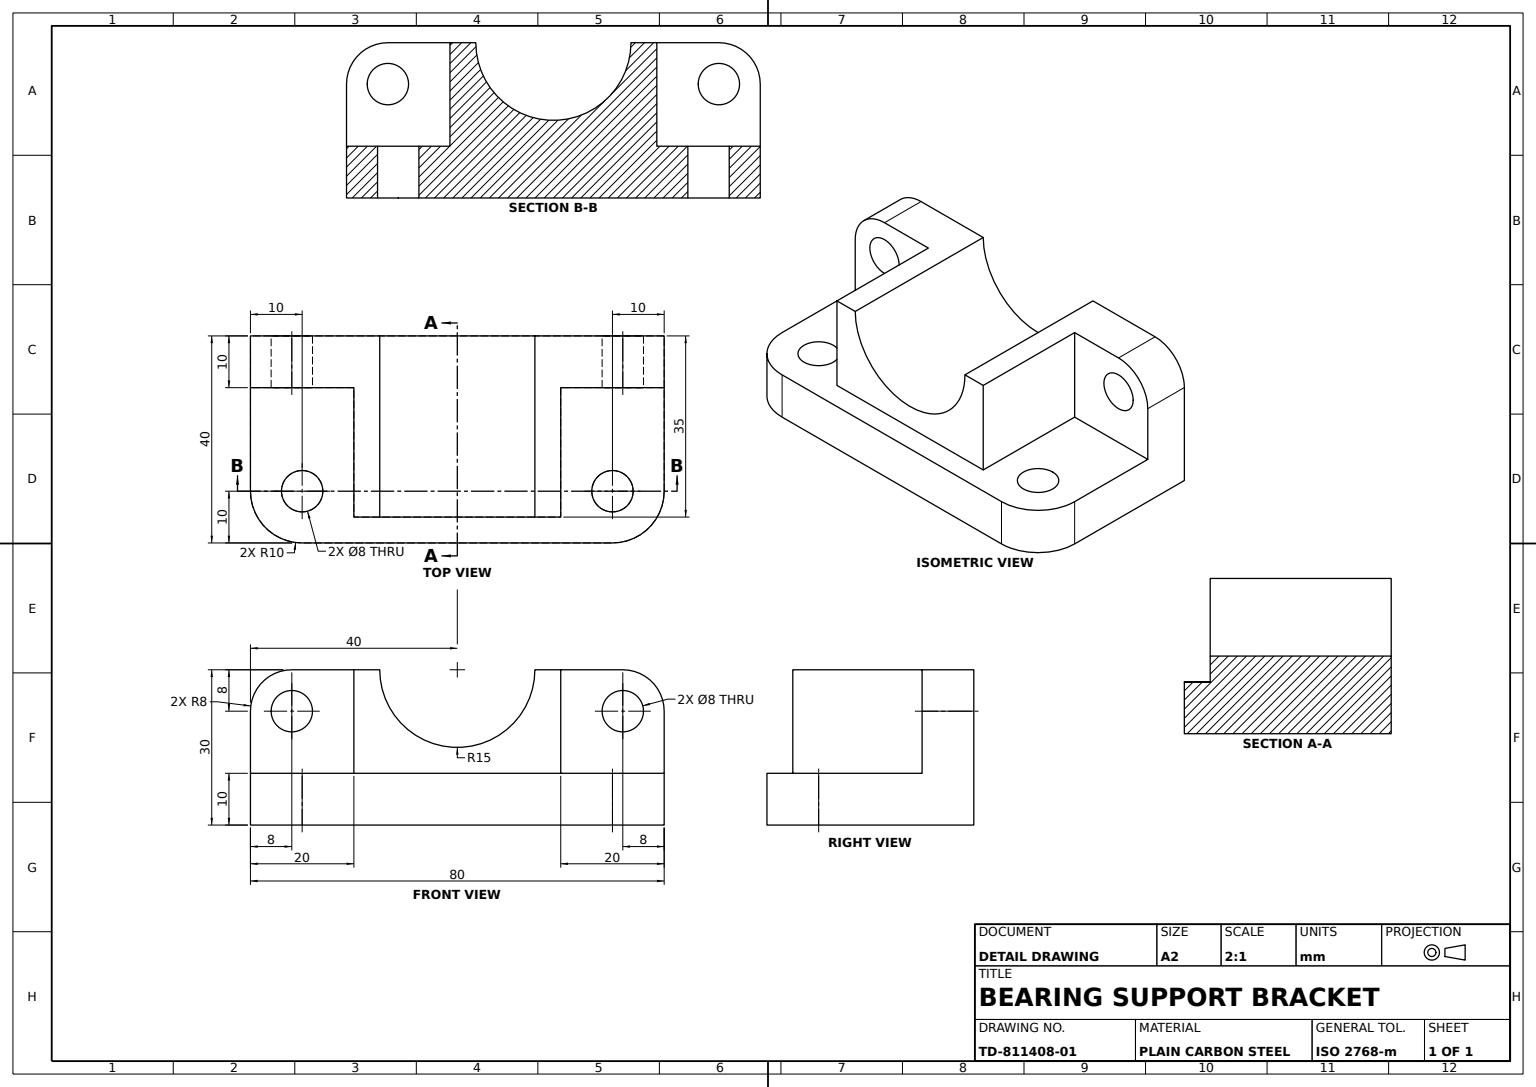
from build123d import *

# Parameters (mm, degrees)
BASE_PLATE_SKETCH_W       = 80
BASE_PLATE_SKETCH_H       = 40
BASE_PLATE_80X40X10_DEPTH = 10
BASE_CORNER_FILLETS_R10_R = 10
SADDLE_BLOCK_DEPTH        = 35
LUG_PROFILE_SKETCH_W      = 20
LUG_PROFILE_SKETCH_H      = 20
UPRIGHT_LUGS_DEPTH        = 10
LUG_TOP_FILLETS_R8_R      = 8
LUG_HOLE_SKETCH_R         = 4
LUG_HOLES_8_DEPTH         = 62
BASE_HOLE_SKETCH_R        = 4
BASE_HOLES_8_DEPTH        = 62


with BuildPart() as part:
    # Base Plate Sketch → Base Plate 80x40x10 (new body)
    with BuildSketch(Plane(origin=(0, 0, 0), x_dir=(1, 0, 0), z_dir=(0, 1, 0))):
        Rectangle(BASE_PLATE_SKETCH_W, BASE_PLATE_SKETCH_H)
    extrude(amount=BASE_PLATE_80X40X10_DEPTH)

    # Base Corner Fillets R10
    base_corner_fillets_r10_edges = [part.edges().sort_by_distance(p)[0] for p in [
        (40, 5, 20),
        (-40, 5, 20),
    ]]
    fillet(base_corner_fillets_r10_edges, radius=BASE_CORNER_FILLETS_R10_R)

    # Saddle Block Sketch → Saddle Block (add)
    with BuildSketch(Plane(origin=(0, 0, -20), x_dir=(-1, 0, 0), z_dir=(0, 0, -1))):
        with BuildLine():
            Line((-20, 10), (20, 10))
            Line((20, 10), (20, 30))
            Line((20, 30), (15, 30))
            ThreePointArc((15, 30), (0, 15), (-15, 30))
            Line((-15, 30), (-20, 30))
            Line((-20, 30), (-20, 10))
        make_face()
    extrude(amount=-SADDLE_BLOCK_DEPTH)

    # Lug Profile Sketch → Upright Lugs (add)
    with BuildSketch(Plane(origin=(0, 0, -20), x_dir=(-1, 0, 0), z_dir=(0, 0, -1))):
        with Locations((-30, 20)):
            Rectangle(LUG_PROFILE_SKETCH_W, LUG_PROFILE_SKETCH_H)
        with Locations((30, 20)):
            Rectangle(LUG_PROFILE_SKETCH_W, LUG_PROFILE_SKETCH_H)
    extrude(amount=-UPRIGHT_LUGS_DEPTH)

    # Lug Top Fillets R8
    lug_top_fillets_r8_edges = [part.edges().sort_by_distance(p)[0] for p in [
        (40, 30, -15),
        (-40, 30, -15),
    ]]
    fillet(lug_top_fillets_r8_edges, radius=LUG_TOP_FILLETS_R8_R)

    # Lug Hole Sketch → Lug Holes Ø8 (cut)
    with BuildSketch(Plane(origin=(0, 0, -20), x_dir=(-1, 0, 0), z_dir=(0, 0, -1))):
        with Locations((32, 22)):
            Circle(LUG_HOLE_SKETCH_R)
        with Locations((-32, 22)):
            Circle(LUG_HOLE_SKETCH_R)
    extrude(amount=-LUG_HOLES_8_DEPTH, mode=Mode.SUBTRACT)

    # Base Hole Sketch → Base Holes Ø8 (cut)
    with BuildSketch(Plane(origin=(0, 10, 0), x_dir=(1, 0, 0), z_dir=(0, 1, 0))):
        with Locations(Location((-30, -10, 0), (0, 0, 270))):
            Circle(BASE_HOLE_SKETCH_R)
        with Locations(Location((30, -10, 0), (0, 0, 270))):
            Circle(BASE_HOLE_SKETCH_R)
    extrude(amount=-BASE_HOLES_8_DEPTH, mode=Mode.SUBTRACT)


solid = part.part
